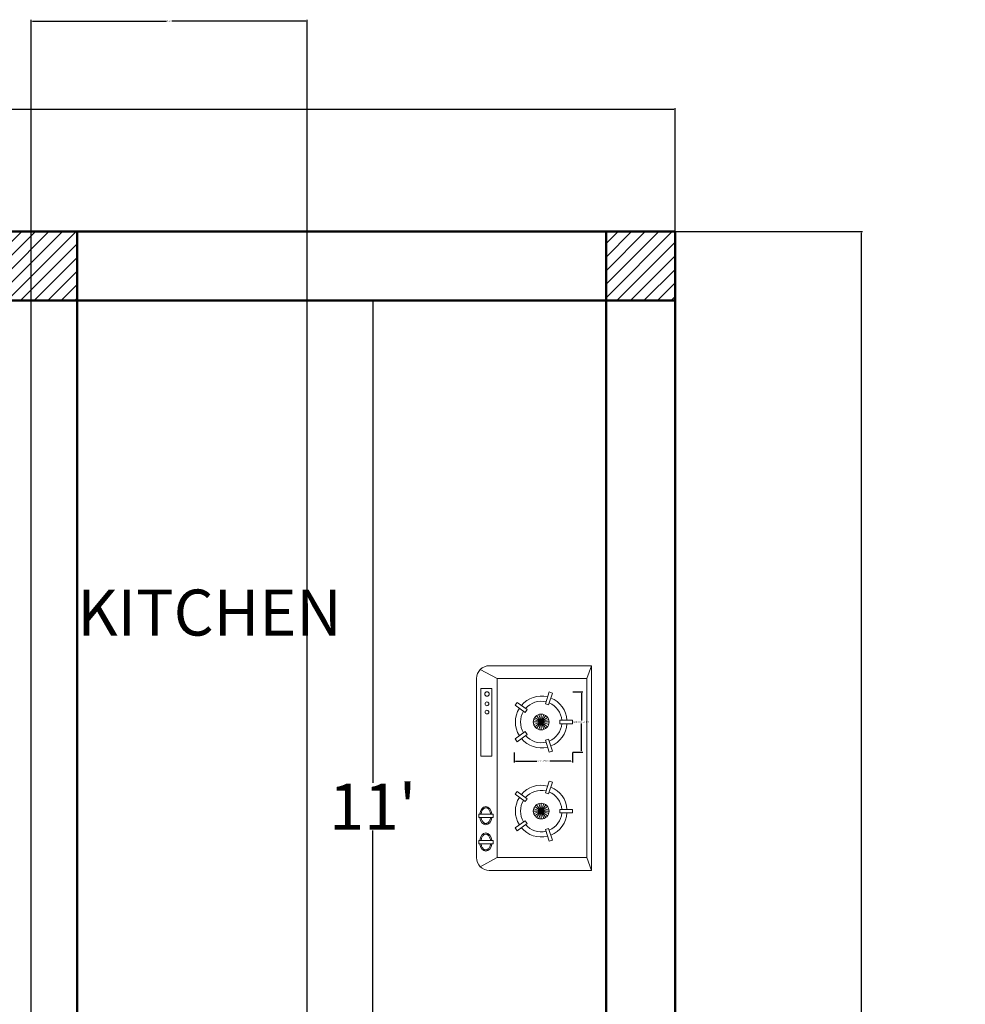
# Model space of a CAD drawing. Units: inches. Extents: x 0 to 281, y -535 to 46.
# Tile 22 of 22: x 158 to 281, y -82 to 46. Entities that reach past the tile are written whole.
import ezdxf

# ---------------------------------------------------------------- set-up
doc = ezdxf.new("R2010")
doc.units = ezdxf.units.IN
doc.header["$MEASUREMENT"] = 0
for name, color, linetype, lineweight in [('A-ANNO-DIMS', 2, 'Continuous', 18), ('A-AREA-IDEN', 7, 'Continuous', 25), ('A-COLS-PATT', 152, 'Continuous', 13), ('A-EQPM', 9, 'Continuous', 18), ('A-WALL', 7, 'Continuous', 50)]:
    doc.layers.add(name, color=color, linetype=linetype, lineweight=lineweight)
doc.styles.get("Standard").update_dxf_attribs({"font": 'arial.ttf'})
doc.dimstyles.get("Standard").update_dxf_attribs({"dimtxt": 0.18, "dimasz": 0.18, "dimexe": 0.18, "dimexo": 0.0625, "dimgap": 0.09, "dimtad": 0, "dimtih": 1, "dimtoh": 1, "dimdec": 0, "dimzin": 0, "dimdsep": 46, "dimlunit": 3, "dimtxsty": 'Standard', "dimcen": 0.09, "dimadec": 0, "dimazin": 0, "dimtfac": 1, "dimtdec": 0, "dimtofl": 0, "dimtmove": 0, "dimatfit": 3, "dimfxl": 1, "dimtolj": 1, "dimtzin": 0, "dimarcsym": 0})

# ---------------------------------------------------------------- blocks, each defined once
blk = doc.blocks.new('*D3')
at = {"layer": 'A-ANNO-DIMS', "color": 0, "lineweight": -2, "transparency": 16777216}
for p, q in [((204.02, 9.41), (204.02, -53.31)), ((204.08, 9.59), (204.2, 9.59)), ((204.02, -122.23), (204.02, -59.51)), ((204.08, -122.41), (204.2, -122.41))]:
    blk.add_line(p, q, dxfattribs=at)
at = {"layer": 'A-ANNO-DIMS', "color": 0, "transparency": 16777216}
for points in [[(203.99, 9.41), (204.05, 9.41), (204.02, 9.59)], [(203.99, -122.23), (204.05, -122.23), (204.02, -122.41)]]:
    blk.add_solid(points, dxfattribs=at)
at = {"layer": 'Defpoints', "color": 0, "transparency": 16777216}
for p in [(204.02, 9.59), (204.02, -122.41), (204.02, -122.41)]:
    blk.add_point(p, dxfattribs=at)
at = {"layer": 'A-ANNO-DIMS', "color": 0, "transparency": 16777216, "insert": (204.02, -56.41), "char_height": 6, "attachment_point": 5}
blk.add_mtext("\\A1;11'", dxfattribs=at)
blk = doc.blocks.new('*D17')
at = {"layer": 'A-ANNO-DIMS', "color": 0, "lineweight": -2, "transparency": 16777216}
for p, q in [((27.46, 18.65), (27.46, 34.69)), ((243.46, 18.65), (243.46, 34.69)), ((27.64, 34.51), (130.56, 34.51)), ((243.28, 34.51), (140.36, 34.51))]:
    blk.add_line(p, q, dxfattribs=at)
at = {"layer": 'A-ANNO-DIMS', "color": 0, "transparency": 16777216}
for points in [[(27.64, 34.54), (27.64, 34.48), (27.46, 34.51)], [(243.28, 34.54), (243.28, 34.48), (243.46, 34.51)]]:
    blk.add_solid(points, dxfattribs=at)
at = {"layer": 'Defpoints', "color": 0, "transparency": 16777216}
for p in [(243.46, 34.51), (27.46, 18.59), (243.46, 18.59)]:
    blk.add_point(p, dxfattribs=at)
at = {"layer": 'A-ANNO-DIMS', "color": 0, "transparency": 16777216, "insert": (135.46, 34.51), "char_height": 6, "attachment_point": 5}
blk.add_mtext("\\A1;18'", dxfattribs=at)
blk = doc.blocks.new('*D18')
at = {"layer": 'A-ANNO-DIMS', "color": 0, "lineweight": -2, "transparency": 16777216}
for p, q in [((243.52, 18.59), (267.93, 18.59)), ((267.75, 18.41), (267.75, -241.26)), ((267.75, -507.23), (267.75, -247.57)), ((243.52, -507.41), (267.93, -507.41))]:
    blk.add_line(p, q, dxfattribs=at)
at = {"layer": 'A-ANNO-DIMS', "color": 0, "transparency": 16777216}
for points in [[(267.72, 18.41), (267.78, 18.41), (267.75, 18.59)], [(267.72, -507.23), (267.78, -507.23), (267.75, -507.41)]]:
    blk.add_solid(points, dxfattribs=at)
at = {"layer": 'Defpoints', "color": 0, "transparency": 16777216}
for p in [(243.46, 18.59), (243.46, -507.41), (267.75, -507.41)]:
    blk.add_point(p, dxfattribs=at)
at = {"layer": 'A-ANNO-DIMS', "color": 0, "transparency": 16777216, "insert": (267.75, -244.41), "char_height": 6, "attachment_point": 5}
blk.add_mtext('\\A1;43\'-10"', dxfattribs=at)
blk = doc.blocks.new('COOKTOP-BURNER')
for p, q in [((3.95, 6.31), (4.45, 7.85)), ((4.88, 7.71), (4.38, 6.17)), ((4.45, 7.85), (4.88, 7.71)), ((0, 6.12), (0.27, 6.49)), ((0.27, 6.49), (1.58, 5.54)), ((1.31, 5.17), (0, 6.12)), ((1.58, 5.54), (1.31, 5.17)), ((4.38, 6.17), (3.95, 6.31)), ((3.41, 3.93), (2.39, 3.93)), ((3.41, 3.93), (2.44, 4.24)), ((3.41, 3.93), (2.44, 3.61)), ((3.41, 3.93), (2.58, 4.53)), ((3.41, 3.93), (2.58, 3.32)), ((3.41, 3.93), (2.81, 4.76)), ((3.41, 3.93), (2.81, 3.09)), ((3.41, 3.93), (3.1, 4.9)), ((3.41, 3.93), (3.1, 2.95)), ((3.41, 3.93), (3.41, 4.95)), ((3.41, 3.93), (3.73, 4.9)), ((3.41, 3.93), (4.02, 4.76)), ((3.41, 3.93), (4.24, 4.53)), ((3.41, 3.93), (4.39, 4.24)), ((3.41, 3.93), (4.44, 3.93)), ((3.41, 3.93), (3.41, 2.9)), ((3.41, 3.93), (3.73, 2.95)), ((3.41, 3.93), (4.02, 3.09)), ((3.41, 3.93), (4.24, 3.32)), ((3.41, 3.93), (4.39, 3.61)), ((5.85, 3.7), (5.85, 4.15)), ((5.85, 4.15), (7.47, 4.15)), ((7.47, 4.15), (7.47, 3.7)), ((0, 1.73), (1.31, 2.68)), ((1.31, 2.68), (1.58, 2.31)), ((7.47, 3.7), (5.85, 3.7)), ((0.27, 1.36), (0, 1.73)), ((1.58, 2.31), (0.27, 1.36)), ((3.95, 1.54), (4.38, 1.68)), ((4.45, 0), (3.95, 1.54)), ((4.38, 1.68), (4.88, 0.14)), ((4.88, 0.14), (4.45, 0))]:
    blk.add_line(p, q)
blk.add_circle((3.41, 3.93), 1.03)
for radius, start, end in [(3.37, 75.8765, 140.1235), (2.7, 76.8365, 139.1635), (3.37, 3.8765, 68.1235), (3.37, 147.8765, 212.1235), (2.7, 148.8365, 211.1635), (2.7, 4.8365, 67.1635), (2.7, 292.8365, 355.1635), (3.37, 291.8765, 356.1235), (3.37, 219.8765, 284.1235), (2.7, 220.8365, 283.1635)]:
    blk.add_arc((3.41, 3.93), radius, start, end)
blk = doc.blocks.new('*D34')
at = {"layer": 'A-ANNO-DIMS', "color": 0, "lineweight": -2, "transparency": 16777216}
for p, q in [((230.12, -41.44), (231.42, -41.44)), ((231.24, -41.62), (231.24, -45.19)), ((231.24, -49.12), (231.24, -45.55)), ((230.12, -49.3), (231.42, -49.3))]:
    blk.add_line(p, q, dxfattribs=at)
at = {"layer": 'A-ANNO-DIMS', "color": 0, "transparency": 16777216}
for points in [[(231.21, -41.62), (231.27, -41.62), (231.24, -41.44)], [(231.21, -49.12), (231.27, -49.12), (231.24, -49.3)]]:
    blk.add_solid(points, dxfattribs=at)
at = {"layer": 'Defpoints', "color": 0, "transparency": 16777216}
for p in [(230.06, -41.44), (231.24, -41.44), (230.06, -49.3)]:
    blk.add_point(p, dxfattribs=at)
at = {"layer": 'A-ANNO-DIMS', "color": 0, "transparency": 16777216, "insert": (231.24, -45.37), "char_height": 0.18, "attachment_point": 5}
blk.add_mtext('\\A1;BURNER 0\'-8" TYP.', dxfattribs=at)
blk = doc.blocks.new('*D35')
at = {"layer": 'A-ANNO-DIMS', "color": 0, "lineweight": -2, "transparency": 16777216}
for p, q in [((222.46, -49.36), (222.46, -50.65)), ((230.06, -49.36), (230.06, -50.65)), ((222.64, -50.47), (225.41, -50.47)), ((229.88, -50.47), (227.11, -50.47))]:
    blk.add_line(p, q, dxfattribs=at)
at = {"layer": 'A-ANNO-DIMS', "color": 0, "transparency": 16777216}
for points in [[(222.64, -50.44), (222.64, -50.5), (222.46, -50.47)], [(229.88, -50.44), (229.88, -50.5), (230.06, -50.47)]]:
    blk.add_solid(points, dxfattribs=at)
at = {"layer": 'Defpoints', "color": 0, "transparency": 16777216}
for p in [(222.46, -49.3), (230.06, -49.3), (230.06, -50.47)]:
    blk.add_point(p, dxfattribs=at)
at = {"layer": 'A-ANNO-DIMS', "color": 0, "transparency": 16777216, "insert": (226.26, -50.47), "char_height": 0.18, "attachment_point": 5}
blk.add_mtext('\\A1;0\'-7 1/2" TYP.', dxfattribs=at)
blk = doc.blocks.new('*D46')
at = {"layer": 'A-ANNO-DIMS', "color": 0, "lineweight": -2, "transparency": 16777216}
for p, q in [((159.46, -263.35), (159.46, 46.22)), ((159.64, 46.04), (177.13, 46.04)), ((195.28, 46.04), (177.79, 46.04)), ((195.46, -263.35), (195.46, 46.22))]:
    blk.add_line(p, q, dxfattribs=at)
at = {"layer": 'A-ANNO-DIMS', "color": 0, "transparency": 16777216}
for points in [[(159.64, 46.07), (159.64, 46.01), (159.46, 46.04)], [(195.28, 46.07), (195.28, 46.01), (195.46, 46.04)]]:
    blk.add_solid(points, dxfattribs=at)
at = {"layer": 'Defpoints', "color": 0, "transparency": 16777216}
for p in [(195.46, 46.04), (159.46, -263.41), (195.46, -263.41)]:
    blk.add_point(p, dxfattribs=at)
at = {"layer": 'A-ANNO-DIMS', "color": 0, "transparency": 16777216, "insert": (177.46, 46.04), "char_height": 0.18, "attachment_point": 5}
blk.add_mtext('\\A1;3\'-0"', dxfattribs=at)
blk = doc.blocks.new('*D48')
at = {"layer": 'A-ANNO-DIMS', "color": 0, "lineweight": -2, "transparency": 16777216}
for p, q in [((159.46, -392.35), (159.46, 46.22)), ((159.64, 46.04), (177.13, 46.04)), ((195.28, 46.04), (177.79, 46.04)), ((195.46, -392.35), (195.46, 46.22))]:
    blk.add_line(p, q, dxfattribs=at)
at = {"layer": 'A-ANNO-DIMS', "color": 0, "transparency": 16777216}
for points in [[(159.64, 46.07), (159.64, 46.01), (159.46, 46.04)], [(195.28, 46.07), (195.28, 46.01), (195.46, 46.04)]]:
    blk.add_solid(points, dxfattribs=at)
at = {"layer": 'Defpoints', "color": 0, "transparency": 16777216}
for p in [(195.46, 46.04), (159.46, -392.41), (195.46, -392.41)]:
    blk.add_point(p, dxfattribs=at)
at = {"layer": 'A-ANNO-DIMS', "color": 0, "transparency": 16777216, "insert": (177.46, 46.04), "char_height": 0.18, "attachment_point": 5}
blk.add_mtext('\\A1;3\'-0"', dxfattribs=at)

msp = doc.modelspace()

# ---------------------------------------------------------------- hatches: boundary and pattern name
at = {"layer": 'A-COLS-PATT'}
h = msp.add_hatch(dxfattribs=at)
h.set_pattern_fill('ANSI31', color=256, scale=10)
h.paths.add_polyline_path([(36.46, 18.59), (27.46, 18.59), (27.46, 9.59), (36.46, 9.59)])
h.paths.add_polyline_path([(165.46, 18.59), (156.46, 18.59), (156.46, 9.59), (165.46, 9.59)])
h.paths.add_polyline_path([(243.46, 18.59), (234.46, 18.59), (234.46, 9.59), (243.46, 9.59)])
h.paths.add_polyline_path([(243.46, -122.41), (234.46, -122.41), (234.46, -131.41), (243.46, -131.41)])
h.paths.add_polyline_path([(36.46, -122.41), (27.46, -122.41), (27.46, -131.41), (36.46, -131.41)])
h.paths.add_polyline_path([(36.46, -498.41), (27.46, -498.41), (27.46, -507.41), (36.46, -507.41)])
h.paths.add_polyline_path([(243.46, -498.41), (234.46, -498.41), (234.46, -507.41), (243.46, -507.41)])
h.paths.add_polyline_path([(159.46, -498.41), (150.46, -498.41), (150.46, -507.41), (159.46, -507.41)])
h.paths.add_polyline_path([(36.46, -392.41), (27.46, -392.41), (27.46, -401.41), (36.46, -401.41)])
h.paths.add_polyline_path([(159.46, -392.41), (150.46, -392.41), (150.46, -401.41), (159.46, -401.41)])
h.paths.add_polyline_path([(243.46, -392.41), (234.46, -392.41), (234.46, -401.41), (243.46, -401.41)])
h.paths.add_polyline_path([(36.46, -263.41), (27.46, -263.41), (27.46, -272.41), (36.46, -272.41)])
h.paths.add_polyline_path([(243.46, -263.41), (234.46, -263.41), (234.46, -272.41), (243.46, -272.41)])

# ---------------------------------------------------------------- linework, layer by layer
at = {"layer": 'A-EQPM'}
for p, q in [((220.26, -39.7), (218.05, -38.52)), ((232.58, -38.03), (219.23, -38.03)), ((231.95, -39.7), (232.58, -38.03)), ((232.58, -64.73), (232.58, -38.03)), ((217.56, -39.7), (217.56, -63.06)), ((231.95, -39.7), (220.26, -39.7)), ((220.26, -39.7), (220.26, -63.06)), ((231.95, -63.06), (231.95, -39.7)), ((218.13, -49.81), (218.13, -40.98)), ((218.13, -40.98), (219.56, -40.98)), ((219.56, -40.98), (219.56, -49.81)), ((219.56, -49.81), (218.13, -49.81)), ((217.86, -57.39), (219.71, -57.39)), ((217.86, -57.82), (217.86, -57.39)), ((219.71, -57.39), (219.71, -57.82)), ((219.71, -57.82), (217.86, -57.82)), ((217.86, -61.28), (217.86, -60.84)), ((217.86, -60.84), (219.71, -60.84)), ((219.71, -61.28), (217.86, -61.28)), ((219.71, -60.84), (219.71, -61.28)), ((220.26, -63.06), (218.05, -64.24)), ((220.26, -63.06), (231.95, -63.06)), ((231.95, -63.06), (232.58, -64.73)), ((219.23, -64.73), (232.58, -64.73))]:
    msp.add_line(p, q, dxfattribs=at)
for centre, radius in [((218.92, -41.72), 0.296), ((218.92, -43), 0.247), ((218.92, -44.08), 0.247)]:
    msp.add_circle(centre, radius, dxfattribs=at)
for centre, start, end in [((219.23, -39.7), 90, 180), ((219.23, -63.06), 180, 270)]:
    msp.add_arc(centre, 1.67, start, end, dxfattribs=at)
for centre, major_axis, start_param, end_param in [((218.77, -57.58), (0, -1.19), 1.73081, 4.552375), ((218.77, -57.58), (0, 1.19), 1.774361, 4.508825), ((218.77, -61.03), (0, -1.19), 1.73081, 4.552375), ((218.77, -61.03), (0, 1.19), 1.774361, 4.508825)]:
    msp.add_ellipse(centre, major_axis=major_axis, ratio=0.671641, start_param=start_param, end_param=end_param, dxfattribs=at)
for points, knots in [([(219.4, -57.39), (219.39, -57.34), (219.39, -57.3), (219.36, -57.18), (219.34, -57.11), (219.29, -56.98), (219.26, -56.91), (219.19, -56.8), (219.16, -56.76), (219.08, -56.67), (219.04, -56.64), (218.96, -56.59), (218.91, -56.57), (218.84, -56.55), (218.81, -56.55), (218.77, -56.55), (218.73, -56.55), (218.69, -56.55), (218.61, -56.58), (218.57, -56.6), (218.49, -56.66), (218.45, -56.69), (218.37, -56.78), (218.34, -56.83), (218.27, -56.95), (218.24, -57.01), (218.2, -57.15), (218.18, -57.22), (218.16, -57.33), (218.15, -57.36), (218.15, -57.39)], [4.889299, 4.889299, 4.889299, 4.889299, 5.015191, 5.015191, 5.233243, 5.233243, 5.451295, 5.451295, 5.669347, 5.669347, 5.887399, 5.887399, 6.10545, 6.10545, 6.283185, 6.283185, 6.283185, 6.501237, 6.501237, 6.719289, 6.719289, 6.937341, 6.937341, 7.155392, 7.155392, 7.373444, 7.373444, 7.591496, 7.591496, 7.677072, 7.677072, 7.677072, 7.677072]), ([(218.16, -57.82), (218.17, -57.88), (218.18, -57.93), (218.21, -58.06), (218.24, -58.13), (218.3, -58.25), (218.33, -58.31), (218.4, -58.41), (218.44, -58.45), (218.52, -58.52), (218.56, -58.54), (218.64, -58.58), (218.69, -58.6), (218.77, -58.61), (218.81, -58.6), (218.89, -58.59), (218.93, -58.57), (219.01, -58.53), (219.05, -58.5), (219.13, -58.43), (219.17, -58.38), (219.24, -58.28), (219.27, -58.22), (219.33, -58.09), (219.35, -58.02), (219.38, -57.91), (219.39, -57.86), (219.39, -57.82)], [8.079302, 8.079302, 8.079302, 8.079302, 8.245651, 8.245651, 8.463703, 8.463703, 8.681755, 8.681755, 8.899807, 8.899807, 9.117859, 9.117859, 9.33591, 9.33591, 9.553962, 9.553962, 9.772014, 9.772014, 9.990066, 9.990066, 10.208118, 10.208118, 10.426169, 10.426169, 10.644221, 10.644221, 10.770253, 10.770253, 10.770253, 10.770253]), ([(219.4, -60.84), (219.39, -60.8), (219.39, -60.75), (219.36, -60.64), (219.34, -60.57), (219.29, -60.43), (219.26, -60.37), (219.19, -60.26), (219.16, -60.21), (219.08, -60.13), (219.04, -60.1), (218.96, -60.05), (218.91, -60.03), (218.84, -60.01), (218.81, -60.01), (218.77, -60.01), (218.73, -60.01), (218.69, -60.01), (218.61, -60.04), (218.57, -60.06), (218.49, -60.12), (218.45, -60.15), (218.37, -60.24), (218.34, -60.29), (218.27, -60.4), (218.24, -60.47), (218.2, -60.6), (218.18, -60.68), (218.16, -60.78), (218.15, -60.81), (218.15, -60.84)], [4.889299, 4.889299, 4.889299, 4.889299, 5.015191, 5.015191, 5.233243, 5.233243, 5.451295, 5.451295, 5.669347, 5.669347, 5.887399, 5.887399, 6.10545, 6.10545, 6.283185, 6.283185, 6.283185, 6.501237, 6.501237, 6.719289, 6.719289, 6.937341, 6.937341, 7.155392, 7.155392, 7.373444, 7.373444, 7.591496, 7.591496, 7.677072, 7.677072, 7.677072, 7.677072]), ([(218.16, -61.28), (218.17, -61.33), (218.18, -61.39), (218.21, -61.52), (218.24, -61.58), (218.3, -61.71), (218.33, -61.77), (218.4, -61.86), (218.44, -61.91), (218.52, -61.98), (218.56, -62), (218.64, -62.04), (218.69, -62.05), (218.77, -62.06), (218.81, -62.06), (218.89, -62.05), (218.93, -62.03), (219.01, -61.99), (219.05, -61.96), (219.13, -61.88), (219.17, -61.84), (219.24, -61.73), (219.27, -61.68), (219.33, -61.55), (219.35, -61.48), (219.38, -61.36), (219.39, -61.32), (219.39, -61.28)], [8.079302, 8.079302, 8.079302, 8.079302, 8.245651, 8.245651, 8.463703, 8.463703, 8.681755, 8.681755, 8.899807, 8.899807, 9.117859, 9.117859, 9.33591, 9.33591, 9.553962, 9.553962, 9.772014, 9.772014, 9.990066, 9.990066, 10.208118, 10.208118, 10.426169, 10.426169, 10.644221, 10.644221, 10.770253, 10.770253, 10.770253, 10.770253])]:
    msp.add_open_spline(points, degree=3, knots=knots, dxfattribs=at)
at = {"layer": 'A-WALL'}
for p, q in [((27.46, 18.59), (243.46, 18.59)), ((165.46, 18.59), (165.46, -131.41)), ((234.46, 18.59), (234.46, -507.41)), ((243.46, 18.59), (243.46, -507.41)), ((27.46, 9.59), (243.46, 9.59))]:
    msp.add_line(p, q, dxfattribs=at)

# ---------------------------------------------------------------- block references
at = {"layer": 'A-EQPM'}
for p in [(222.59, -49.3), (222.59, -60.92)]:
    msp.add_blockref('COOKTOP-BURNER', p, dxfattribs=at)

# ---------------------------------------------------------------- texts
at = {"layer": 'A-AREA-IDEN', "insert": (165.46, -28.1), "char_height": 6, "attachment_point": 1}
msp.add_mtext('KITCHEN', dxfattribs=at)

# ---------------------------------------------------------------- dimensions: what is measured, and where the dimension line sits
at = {"layer": 'A-ANNO-DIMS'}
for base, p1, p2, override, picture, middle in [((195.46, 46.04), (159.46, -263.41), (195.46, -263.41), {"dimdec": 1, "dimlfac": 1, "dimrnd": 0, "dimzin": 1, "dimdsep": 46, "dimlunit": 4, "dimfrac": 2}, '*D46', (177.46, 46.04)), ((195.46, 46.04), (159.46, -392.41), (195.46, -392.41), {"dimdec": 1, "dimlfac": 1, "dimrnd": 0, "dimzin": 1, "dimdsep": 46, "dimlunit": 4, "dimfrac": 2}, '*D48', (177.46, 46.04)), ((243.46, 34.51), (27.46, 18.59), (243.46, 18.59), {"dimtxt": 6, "dimclrd": 0, "dimclre": 0, "dimclrt": 0}, '*D17', (135.46, 34.51))]:
    dim = msp.add_linear_dim(base=base, p1=p1, p2=p2, dimstyle='Standard', override=override, dxfattribs=at)
    dim.commit()
    dim.dimension.update_dxf_attribs({"geometry": picture, "text_midpoint": middle})
for base, p1, p2, picture, middle in [((267.75, -507.41), (243.46, 18.59), (243.46, -507.41), '*D18', (267.75, -244.41)), ((204.02, -122.41), (204.02, 9.59), (204.02, -122.41), '*D3', (204.02, -56.41))]:
    dim = msp.add_linear_dim(base=base, p1=p1, p2=p2, angle=90, dimstyle='Standard', override={"dimtxt": 6, "dimclrd": 0, "dimclre": 0, "dimclrt": 0}, dxfattribs=at)
    dim.commit()
    dim.dimension.update_dxf_attribs({"geometry": picture, "text_midpoint": middle})
dim = msp.add_linear_dim(base=(231.24, -41.44), p1=(230.06, -49.3), p2=(230.06, -41.44), angle=90, text='BURNER <> TYP.', dimstyle='Standard', override={"dimdec": 1, "dimlfac": 1, "dimrnd": 0, "dimzin": 1, "dimdsep": 46, "dimlunit": 4, "dimfrac": 2}, dxfattribs=at)
dim.commit()
dim.dimension.update_dxf_attribs({"geometry": '*D34', "text_midpoint": (231.24, -45.37)})
dim = msp.add_linear_dim(base=(230.06, -50.47), p1=(222.46, -49.3), p2=(230.06, -49.3), text='<> TYP.', dimstyle='Standard', override={"dimdec": 1, "dimlfac": 1, "dimrnd": 0, "dimzin": 1, "dimdsep": 46, "dimlunit": 4, "dimfrac": 2}, dxfattribs=at)
dim.commit()
dim.dimension.update_dxf_attribs({"geometry": '*D35', "text_midpoint": (226.26, -50.47)})

doc.saveas('drawing.dxf')
